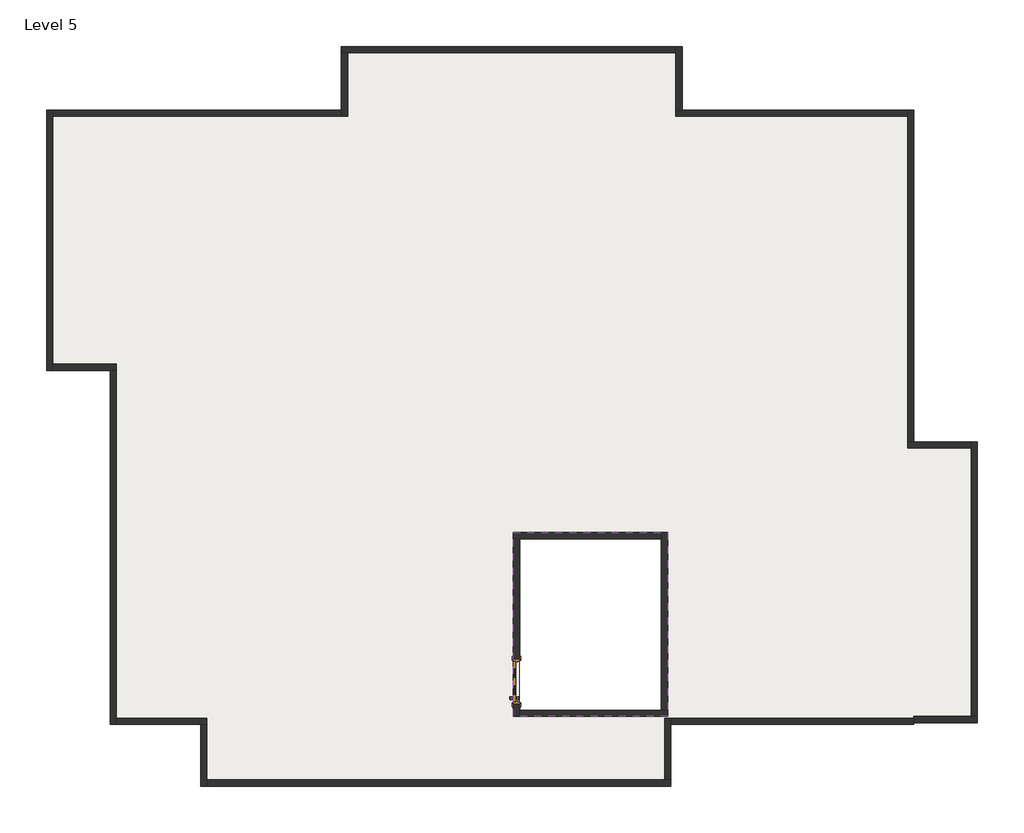
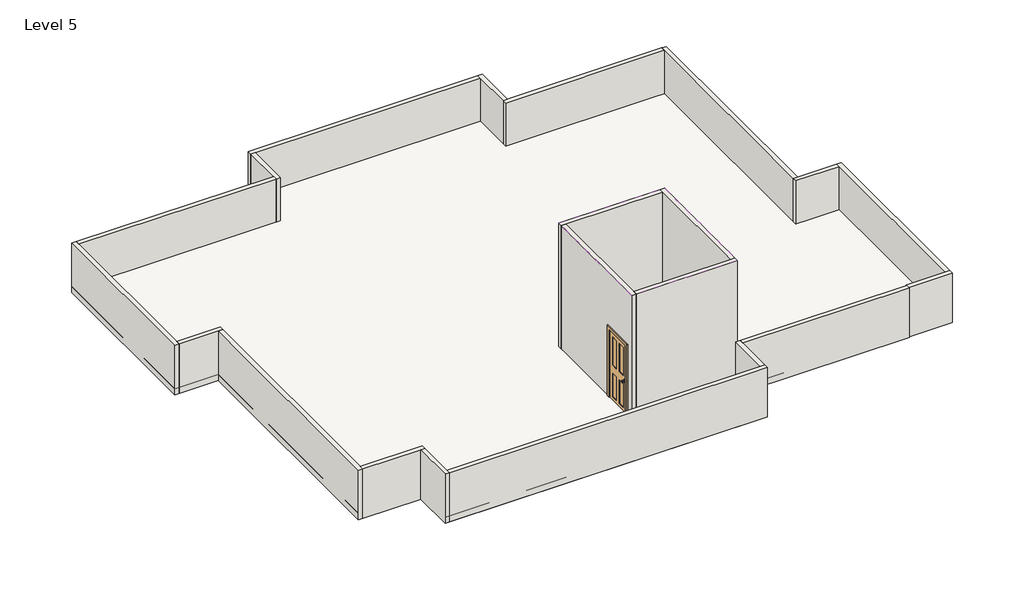
# One storey: 21 walls, 1 covering, 1 door, 1 slab.
"""IFC4 building model written with IfcOpenShell, lengths in millimetres."""

from ifc_helpers import new_model, si_unit, frame, origin, place, context, project, spatial, polyline, outline, extrude, faceted_brep, transform, mapped, element, save
from components import door_7e1124f1

model = new_model("IFC4")

# Units and contexts
model_context = context("Model", 3, world=origin())
ifc_project = project(units=[si_unit("LENGTHUNIT", "METRE", prefix="MILLI")], contexts=[model_context])

# Site, building, storey
site = spatial("IfcSite", under=ifc_project)
building = spatial("IfcBuilding", under=site)
storey = spatial("IfcBuildingStorey", under=building, Name="Level 5", Elevation=12801.6)

# Covering
placement = place(None, origin())
element("IfcCovering", 1, ObjectType="Plain", at=placement, inside=storey, context=model_context, shape_type="SweptSolid", body=[
    extrude(outline(polyline([(-9375.9794909, -1406.3618509), (-9375.9794909, -4352.7618509), (-11843.7794909, -4352.7618509), (-11843.7794909, -1406.3618509), (-9375.9794909, -1406.3618509)])), frame((0.0, 0.0, 16002.0), z_axis=(0.0, 0.0, 1.0), x_axis=(1.0, 0.0, 0.0)), (0.0, 0.0, 1.0), 57.0),
])

# Door
door_shape = door_7e1124f1(model_context)
element("IfcDoor", 2, ObjectType="M_Door-Interior-Single-4_Panel-Wood : 2'2\"", at=placement, inside=storey, context=model_context, shape_type="MappedRepresentation", body=[
    mapped(door_shape, transform((-11796.1544909, -3794.3618509, 12801.6), x_axis=(0.0, 1.0, 0.0), y_axis=(-1.0, 0.0, 0.0), z_axis=(0.0, 0.0, 1.0))),
])

# Slab
element("IfcSlab", 3, ObjectType="Generic 150mm", at=placement, inside=storey, context=model_context, shape_type="SweptSolid", body=[
    extrude(outline(polyline([(-18291.3794909, 1184.4381491), (-19307.3794909, 1184.4381491), (-19307.3794909, 5350.0381491), (-14596.2721539, 5350.0381491), (-14596.2721539, 6366.0381491), (-9142.3367869, 6366.0381491), (-9142.3367869, 5350.0381491), (-5438.9794909, 5350.0381491), (-5438.9794909, 41.4381491), (-4422.9794909, 41.4381491), (-4422.9794909, -4454.3618509), (-5438.9794909, -4454.3618509), (-5438.9794909, -4479.7618509), (-9325.1794909, -4479.7618509), (-9325.1794909, -5470.3618509), (-16843.5794909, -5470.3618509), (-16843.5794909, -4479.7618509), (-18291.3794909, -4479.7618509), (-18291.3794909, 1184.4381491)]), holes=[polyline([(-11738.1794909, -1507.9618509), (-11738.1794909, -4251.1618509), (-9477.5794909, -4251.1618509), (-9477.5794909, -1507.9618509), (-11738.1794909, -1507.9618509)])]), frame((0.0, 0.0, 12804.0), z_axis=(0.0, 0.0, 1.0), x_axis=(1.0, 0.0, 0.0)), (0.0, 0.0, 1.0), 150.0),
])

# Walls
element("IfcWall", 4, ObjectType="Generic - 4\"", at=placement, inside=storey, context=model_context, shape_type="Brep", body=[
    faceted_brep([(-19307.3794909, 5350.0381491, 12801.6), (-19307.3794909, 1184.4381491, 12801.6), (-19307.3794909, 1184.4381491, 14020.8), (-19307.3794909, 5350.0381491, 14020.8), (-19205.7794909, 5350.0381491, 12801.6), (-19205.7794909, 5350.0381491, 14020.8), (-19205.7794909, 5248.4381491, 14020.8), (-19205.7794909, 1286.0381491, 14020.8), (-19205.7794909, 1184.4381491, 14020.8), (-19205.7794909, 1184.4381491, 12801.6), (-19205.7794909, 1286.0381491, 12801.6), (-19205.7794909, 5248.4381491, 12801.6)], [[[0, 1, 2, 3]], [[4, 5, 6, 7, 8, 9, 10, 11]], [[1, 0, 4, 11, 10, 9]], [[3, 2, 8, 7, 6, 5]], [[2, 1, 9, 8]], [[0, 3, 5, 4]]]),
])
element("IfcWall", 5, ObjectType="Generic - 4\"", at=placement, inside=storey, context=model_context, shape_type="Brep", body=[
    faceted_brep([(-19205.7794909, 1184.4381491, 12801.6), (-18291.3794909, 1184.4381491, 12801.6), (-18189.7794909, 1184.4381491, 12801.6), (-18189.7794909, 1184.4381491, 14020.8), (-18291.3794909, 1184.4381491, 14020.8), (-19205.7794909, 1184.4381491, 14020.8), (-19205.7794909, 1286.0381491, 12801.6), (-19205.7794909, 1286.0381491, 14020.8), (-18189.7794909, 1286.0381491, 14020.8), (-18189.7794909, 1286.0381491, 12801.6)], [[[0, 1, 2, 3, 4, 5]], [[6, 7, 8, 9]], [[2, 1, 0, 6, 9]], [[5, 4, 3, 8, 7]], [[0, 5, 7, 6]], [[3, 2, 9, 8]]]),
])
element("IfcWall", 6, ObjectType="Generic - 4\"", at=placement, inside=storey, context=model_context, shape_type="Brep", body=[
    faceted_brep([(-18291.3794909, 1184.4381491, 12801.6), (-18291.3794909, -4479.7618509, 12801.6), (-18291.3794909, -4479.7618509, 14020.8), (-18291.3794909, 1184.4381491, 14020.8), (-18189.7794909, 1184.4381491, 12801.6), (-18189.7794909, 1184.4381491, 14020.8), (-18189.7794909, -4378.1618509, 14020.8), (-18189.7794909, -4479.7618509, 14020.8), (-18189.7794909, -4479.7618509, 12801.6), (-18189.7794909, -4378.1618509, 12801.6)], [[[0, 1, 2, 3]], [[4, 5, 6, 7, 8, 9]], [[1, 0, 4, 9, 8]], [[3, 2, 7, 6, 5]], [[0, 3, 5, 4]], [[2, 1, 8, 7]]]),
])
element("IfcWall", 7, ObjectType="Generic - 4\"", at=placement, inside=storey, context=model_context, shape_type="Brep", body=[
    faceted_brep([(-18189.7794909, -4479.7618509, 12801.6), (-16843.5794909, -4479.7618509, 12801.6), (-16741.9794909, -4479.7618509, 12801.6), (-16741.9794909, -4479.7618509, 14020.8), (-16843.5794909, -4479.7618509, 14020.8), (-18189.7794909, -4479.7618509, 14020.8), (-18189.7794909, -4378.1618509, 12801.6), (-18189.7794909, -4378.1618509, 14020.8), (-16741.9794909, -4378.1618509, 14020.8), (-16741.9794909, -4378.1618509, 12801.6)], [[[0, 1, 2, 3, 4, 5]], [[6, 7, 8, 9]], [[2, 1, 0, 6, 9]], [[5, 4, 3, 8, 7]], [[0, 5, 7, 6]], [[3, 2, 9, 8]]]),
])
element("IfcWall", 8, ObjectType="Generic - 4\"", at=placement, inside=storey, context=model_context, shape_type="Brep", body=[
    faceted_brep([(-16843.5794909, -4479.7618509, 12801.6), (-16843.5794909, -5470.3618509, 12801.6), (-16843.5794909, -5470.3618509, 14020.8), (-16843.5794909, -4479.7618509, 14020.8), (-16741.9794909, -4479.7618509, 12801.6), (-16741.9794909, -4479.7618509, 14020.8), (-16741.9794909, -5368.7618509, 14020.8), (-16741.9794909, -5470.3618509, 14020.8), (-16741.9794909, -5470.3618509, 12801.6), (-16741.9794909, -5368.7618509, 12801.6)], [[[0, 1, 2, 3]], [[4, 5, 6, 7, 8, 9]], [[1, 0, 4, 9, 8]], [[3, 2, 7, 6, 5]], [[0, 3, 5, 4]], [[2, 1, 8, 7]]]),
])
element("IfcWall", 9, ObjectType="Generic - 4\"", at=placement, inside=storey, context=model_context, shape_type="Brep", body=[
    faceted_brep([(-16741.9794909, -5470.3618509, 12801.6), (-9325.1794909, -5470.3618509, 12801.6), (-9325.1794909, -5470.3618509, 14020.8), (-16741.9794909, -5470.3618509, 14020.8), (-16741.9794909, -5368.7618509, 12801.6), (-16741.9794909, -5368.7618509, 14020.8), (-9426.7794909, -5368.7618509, 14020.8), (-9325.1794909, -5368.7618509, 14020.8), (-9325.1794909, -5368.7618509, 12801.6), (-9426.7794909, -5368.7618509, 12801.6)], [[[0, 1, 2, 3]], [[4, 5, 6, 7, 8, 9]], [[1, 0, 4, 9, 8]], [[3, 2, 7, 6, 5]], [[0, 3, 5, 4]], [[2, 1, 8, 7]]]),
])
element("IfcWall", 10, ObjectType="Generic - 4\"", at=placement, inside=storey, context=model_context, shape_type="Brep", body=[
    faceted_brep([(-9325.1794909, -5368.7618509, 12801.6), (-9325.1794909, -4479.7618509, 12801.6), (-9325.1794909, -4378.1618509, 12801.6), (-9325.1794909, -4378.1618509, 14020.8), (-9325.1794909, -4479.7618509, 14020.8), (-9325.1794909, -5368.7618509, 14020.8), (-9426.7794909, -5368.7618509, 12801.6), (-9426.7794909, -5368.7618509, 14020.8), (-9426.7794909, -4378.1618509, 14020.8), (-9426.7794909, -4378.1618509, 12801.6)], [[[0, 1, 2, 3, 4, 5]], [[6, 7, 8, 9]], [[2, 1, 0, 6, 9]], [[5, 4, 3, 8, 7]], [[0, 5, 7, 6]], [[3, 2, 9, 8]]]),
])
element("IfcWall", 11, ObjectType="Generic - 4\"", at=placement, inside=storey, context=model_context, shape_type="Brep", body=[
    faceted_brep([(-9325.1794909, -4479.7618509, 12801.6), (-5438.9794909, -4479.7618509, 12801.6), (-5438.9794909, -4479.7618509, 14020.8), (-9325.1794909, -4479.7618509, 14020.8), (-9325.1794909, -4378.1618509, 12801.6), (-9325.1794909, -4378.1618509, 14020.8), (-5438.9794909, -4378.1618509, 14020.8), (-5438.9794909, -4378.1618509, 12801.6), (-5438.9794909, -4454.3618509, 12801.6), (-5438.9794909, -4454.3618509, 14020.8)], [[[0, 1, 2, 3]], [[4, 5, 6, 7]], [[1, 0, 4, 7, 8]], [[2, 1, 8, 7, 6, 9]], [[3, 2, 9, 6, 5]], [[0, 3, 5, 4]]]),
])
element("IfcWall", 12, ObjectType="Generic - 4\"", at=placement, inside=storey, context=model_context, shape_type="Brep", body=[
    faceted_brep([(-5438.9794909, -4454.3618509, 12801.6), (-4422.9794909, -4454.3618509, 12801.6), (-4422.9794909, -4454.3618509, 14020.8), (-5438.9794909, -4454.3618509, 14020.8), (-5438.9794909, -4352.7618509, 12801.6), (-5438.9794909, -4352.7618509, 14020.8), (-4524.5794909, -4352.7618509, 14020.8), (-4422.9794909, -4352.7618509, 14020.8), (-4422.9794909, -4352.7618509, 12801.6), (-4524.5794909, -4352.7618509, 12801.6), (-5438.9794909, -4378.1618509, 12801.6), (-5438.9794909, -4378.1618509, 14020.8)], [[[0, 1, 2, 3]], [[4, 5, 6, 7, 8, 9]], [[1, 0, 10, 4, 9, 8]], [[3, 2, 7, 6, 5, 11]], [[0, 3, 11, 5, 4, 10]], [[2, 1, 8, 7]]]),
])
element("IfcWall", 13, ObjectType="Generic - 4\"", at=placement, inside=storey, context=model_context, shape_type="Brep", body=[
    faceted_brep([(-4422.9794909, -4352.7618509, 12801.6), (-4422.9794909, 41.4381491, 12801.6), (-4422.9794909, 41.4381491, 14020.8), (-4422.9794909, -4352.7618509, 14020.8), (-4524.5794909, -4352.7618509, 12801.6), (-4524.5794909, -4352.7618509, 14020.8), (-4524.5794909, -60.1618509, 14020.8), (-4524.5794909, 41.4381491, 14020.8), (-4524.5794909, 41.4381491, 12801.6), (-4524.5794909, -60.1618509, 12801.6)], [[[0, 1, 2, 3]], [[4, 5, 6, 7, 8, 9]], [[1, 0, 4, 9, 8]], [[3, 2, 7, 6, 5]], [[0, 3, 5, 4]], [[2, 1, 8, 7]]]),
])
element("IfcWall", 14, ObjectType="Generic - 4\"", at=placement, inside=storey, context=model_context, shape_type="Brep", body=[
    faceted_brep([(-4524.5794909, 41.4381491, 12801.6), (-5438.9794909, 41.4381491, 12801.6), (-5540.5794909, 41.4381491, 12801.6), (-5540.5794909, 41.4381491, 14020.8), (-5438.9794909, 41.4381491, 14020.8), (-4524.5794909, 41.4381491, 14020.8), (-4524.5794909, -60.1618509, 12801.6), (-4524.5794909, -60.1618509, 14020.8), (-5540.5794909, -60.1618509, 14020.8), (-5540.5794909, -60.1618509, 12801.6)], [[[0, 1, 2, 3, 4, 5]], [[6, 7, 8, 9]], [[2, 1, 0, 6, 9]], [[5, 4, 3, 8, 7]], [[0, 5, 7, 6]], [[3, 2, 9, 8]]]),
])
element("IfcWall", 15, ObjectType="Generic - 4\"", at=placement, inside=storey, context=model_context, shape_type="Brep", body=[
    faceted_brep([(-5438.9794909, 41.4381491, 12801.6), (-5438.9794909, 5350.0381491, 12801.6), (-5438.9794909, 5350.0381491, 14020.8), (-5438.9794909, 41.4381491, 14020.8), (-5540.5794909, 41.4381491, 12801.6), (-5540.5794909, 41.4381491, 14020.8), (-5540.5794909, 5248.4381491, 14020.8), (-5540.5794909, 5350.0381491, 14020.8), (-5540.5794909, 5350.0381491, 12801.6), (-5540.5794909, 5248.4381491, 12801.6)], [[[0, 1, 2, 3]], [[4, 5, 6, 7, 8, 9]], [[1, 0, 4, 9, 8]], [[3, 2, 7, 6, 5]], [[0, 3, 5, 4]], [[2, 1, 8, 7]]]),
])
element("IfcWall", 16, ObjectType="Generic - 4\"", at=placement, inside=storey, context=model_context, shape_type="Brep", body=[
    faceted_brep([(-5540.5794909, 5350.0381491, 12801.6), (-9142.3367869, 5350.0381491, 12801.6), (-9243.9367869, 5350.0381491, 12801.6), (-9243.9367869, 5350.0381491, 14020.8), (-9142.3367869, 5350.0381491, 14020.8), (-5540.5794909, 5350.0381491, 14020.8), (-5540.5794909, 5248.4381491, 12801.6), (-5540.5794909, 5248.4381491, 14020.8), (-9243.9367869, 5248.4381491, 14020.8), (-9243.9367869, 5248.4381491, 12801.6)], [[[0, 1, 2, 3, 4, 5]], [[6, 7, 8, 9]], [[2, 1, 0, 6, 9]], [[5, 4, 3, 8, 7]], [[0, 5, 7, 6]], [[3, 2, 9, 8]]]),
])
element("IfcWall", 17, ObjectType="Generic - 4\"", at=placement, inside=storey, context=model_context, shape_type="Brep", body=[
    faceted_brep([(-9142.3367869, 5350.0381491, 12801.6), (-9142.3367869, 6366.0381491, 12801.6), (-9142.3367869, 6366.0381491, 14020.8), (-9142.3367869, 5350.0381491, 14020.8), (-9243.9367869, 5350.0381491, 12801.6), (-9243.9367869, 5350.0381491, 14020.8), (-9243.9367869, 6264.4381491, 14020.8), (-9243.9367869, 6366.0381491, 14020.8), (-9243.9367869, 6366.0381491, 12801.6), (-9243.9367869, 6264.4381491, 12801.6)], [[[0, 1, 2, 3]], [[4, 5, 6, 7, 8, 9]], [[1, 0, 4, 9, 8]], [[3, 2, 7, 6, 5]], [[0, 3, 5, 4]], [[2, 1, 8, 7]]]),
])
element("IfcWall", 18, ObjectType="Generic - 4\"", at=placement, inside=storey, context=model_context, shape_type="Brep", body=[
    faceted_brep([(-9243.9367869, 6366.0381491, 12801.6), (-14596.2721539, 6366.0381491, 12801.6), (-14596.2721539, 6366.0381491, 14020.8), (-9243.9367869, 6366.0381491, 14020.8), (-9243.9367869, 6264.4381491, 12801.6), (-9243.9367869, 6264.4381491, 14020.8), (-14494.6721539, 6264.4381491, 14020.8), (-14596.2721539, 6264.4381491, 14020.8), (-14596.2721539, 6264.4381491, 12801.6), (-14494.6721539, 6264.4381491, 12801.6)], [[[0, 1, 2, 3]], [[4, 5, 6, 7, 8, 9]], [[1, 0, 4, 9, 8]], [[3, 2, 7, 6, 5]], [[0, 3, 5, 4]], [[2, 1, 8, 7]]]),
])
element("IfcWall", 19, ObjectType="Generic - 4\"", at=placement, inside=storey, context=model_context, shape_type="Brep", body=[
    faceted_brep([(-14596.2721539, 6264.4381491, 12801.6), (-14596.2721539, 5350.0381491, 12801.6), (-14596.2721539, 5248.4381491, 12801.6), (-14596.2721539, 5248.4381491, 14020.8), (-14596.2721539, 5350.0381491, 14020.8), (-14596.2721539, 6264.4381491, 14020.8), (-14494.6721539, 6264.4381491, 12801.6), (-14494.6721539, 6264.4381491, 14020.8), (-14494.6721539, 5248.4381491, 14020.8), (-14494.6721539, 5248.4381491, 12801.6)], [[[0, 1, 2, 3, 4, 5]], [[6, 7, 8, 9]], [[2, 1, 0, 6, 9]], [[5, 4, 3, 8, 7]], [[0, 5, 7, 6]], [[3, 2, 9, 8]]]),
])
element("IfcWall", 20, ObjectType="Generic - 4\"", at=placement, inside=storey, context=model_context, shape_type="SweptSolid", body=[
    extrude(outline(polyline([(-19205.7794909, 5350.0381491), (-14596.2721539, 5350.0381491), (-14596.2721539, 5248.4381491), (-19205.7794909, 5248.4381491), (-19205.7794909, 5350.0381491)])), frame((0.0, 0.0, 12801.6), z_axis=(0.0, 0.0, 1.0), x_axis=(1.0, 0.0, 0.0)), (0.0, 0.0, 1.0), 1219.2),
])
element("IfcWall", 21, ObjectType="Generic - 4\"", at=placement, inside=storey, context=model_context, shape_type="Brep", body=[
    faceted_brep([(-9375.9794909, -4251.1618509, 12801.6), (-9477.5794909, -4251.1618509, 12801.6), (-11742.1794909, -4251.1618509, 12801.6), (-11742.1794909, -4251.1618509, 16002.0), (-9477.5794909, -4251.1618509, 16002.0), (-9375.9794909, -4251.1618509, 16002.0), (-9375.9794909, -4352.7618509, 12801.6), (-9375.9794909, -4352.7618509, 16002.0), (-11742.1794909, -4352.7618509, 16002.0), (-11742.1794909, -4352.7618509, 12801.6)], [[[0, 1, 2, 3, 4, 5]], [[6, 7, 8, 9]], [[2, 1, 0, 6, 9]], [[5, 4, 3, 8, 7]], [[0, 5, 7, 6]], [[3, 2, 9, 8]]]),
])
element("IfcWall", 22, ObjectType="Generic - 4\"", at=placement, inside=storey, context=model_context, shape_type="Brep", body=[
    faceted_brep([(-9477.5794909, -1406.3618509, 12801.6), (-9477.5794909, -1507.9618509, 12801.6), (-9477.5794909, -4251.1618509, 12801.6), (-9477.5794909, -4251.1618509, 16002.0), (-9477.5794909, -1507.9618509, 16002.0), (-9477.5794909, -1406.3618509, 16002.0), (-9375.9794909, -1406.3618509, 12801.6), (-9375.9794909, -1406.3618509, 16002.0), (-9375.9794909, -4251.1618509, 16002.0), (-9375.9794909, -4251.1618509, 12801.6)], [[[0, 1, 2, 3, 4, 5]], [[6, 7, 8, 9]], [[2, 1, 0, 6, 9]], [[5, 4, 3, 8, 7]], [[0, 5, 7, 6]], [[3, 2, 9, 8]]]),
])
element("IfcWall", 23, ObjectType="Generic - 4\"", at=placement, inside=storey, context=model_context, shape_type="Brep", body=[
    faceted_brep([(-11843.7794909, -1507.9618509, 12801.6), (-11742.1794909, -1507.9618509, 12801.6), (-9477.5794909, -1507.9618509, 12801.6), (-9477.5794909, -1507.9618509, 16002.0), (-11742.1794909, -1507.9618509, 16002.0), (-11843.7794909, -1507.9618509, 16002.0), (-11843.7794909, -1406.3618509, 12801.6), (-11843.7794909, -1406.3618509, 16002.0), (-9477.5794909, -1406.3618509, 16002.0), (-9477.5794909, -1406.3618509, 12801.6)], [[[0, 1, 2, 3, 4, 5]], [[6, 7, 8, 9]], [[2, 1, 0, 6, 9]], [[5, 4, 3, 8, 7]], [[0, 5, 7, 6]], [[3, 2, 9, 8]]]),
])
element("IfcWall", 24, ObjectType="Generic - 4\"", at=placement, inside=storey, context=model_context, shape_type="Brep", body=[
    faceted_brep([(-11742.1794909, -1507.9618509, 16002.0), (-11742.1794909, -4251.1618509, 16002.0), (-11742.1794909, -4352.7618509, 16002.0), (-11742.1794909, -4352.7618509, 12801.6), (-11742.1794909, -4251.1618509, 12801.6), (-11742.1794909, -4149.5618509, 12801.6), (-11742.1794909, -4149.5618509, 14655.4), (-11742.1794909, -3439.1618509, 14655.4), (-11742.1794909, -3439.1618509, 12801.6), (-11742.1794909, -1507.9618509, 12801.6), (-11843.7794909, -4352.7618509, 16002.0), (-11843.7794909, -1507.9618509, 16002.0), (-11843.7794909, -1507.9618509, 12801.6), (-11843.7794909, -3439.1618509, 12801.6), (-11843.7794909, -3439.1618509, 14655.4), (-11843.7794909, -4149.5618509, 14655.4), (-11843.7794909, -4149.5618509, 12801.6), (-11843.7794909, -4352.7618509, 12801.6)], [[[0, 1, 2, 3, 4, 5, 6, 7, 8, 9]], [[10, 11, 12, 13, 14, 15, 16, 17]], [[3, 17, 16, 5, 4]], [[12, 9, 8, 13]], [[2, 1, 0, 11, 10]], [[3, 2, 10, 17]], [[0, 9, 12, 11]], [[7, 14, 13, 8]], [[15, 6, 5, 16]], [[6, 15, 14, 7]]]),
])

save(model, "model.ifc")

# Revit data of these elements
# Type "Plain"
#   built-in parameter 1002203 = 1 (stored number, unit not read)
#   built-in parameter 1002202 = 1 (stored number, unit not read)
#   Layers, outside or top first: 0' - 1.77165" "Metal Stud Layer" (function 1); 0' - 0.47244" "Gypsum Wall Board" (function 1)
# Type "M_Door-Interior-Single-4_Panel-Wood : 2'2\""
#   Type Mark = "43"
#   Assembly Code = "C1020300"
#   Analytic Construction = "Wooden"
#   Top Rail = 0' - 4.72441"
#   Thickness = 0' - 1.37795"
#   Thermal Resistance (R) = 0.455703 (m²·K)/W
#   Swing Angle [instance default] = 90.00°
#   Stiles = 0' - 4.72441"
#   Rough Width = 2' - 3.9685"
#   Rough Height = 6' - 0.98425"
#   Mullion = 0' - 4.52756"
#   Lock Rail = 0' - 7.87402"
#   Height = 6' - 0"
#   Width = 2' - 2"
#   Heat Transfer Coefficient (U) = 2.19465 W/(m²·K)
#   Bottom Rail = 0' - 9.05512"
#   Trim Material = Cherry
#   Panel Material = Cherry
#   Frame Material = Cherry
#   Door Handle Material = Aluminum
#   Visual Light Transmittance = 0
#   Solar Heat Gain Coefficient = 0
#   Wall Closure = (empty or 0)
#   Function = (empty or 0)
# Type "Generic 150mm"
#   Function = 0
#   Layers, outside or top first: 0' - 5.90551" no material (function 1)
# Type "Generic - 4\""
#   Layers, outside or top first: 0' - 4" no material (function 1)
# Element 1 (IfcCovering, "Plain")
#   Height Offset From Level = 10' - 6"
#   Phase Created = New Construction
#   Materials on its faces: "Gypsum Wall Board", "Metal Stud Layer"
# Element 2 (IfcDoor, "M_Door-Interior-Single-4_Panel-Wood : 2'2\"")
#   Swing Angle = 90.00°
#   Phase Created = New Construction
#   Materials on its faces: "Cherry", "Aluminum"
# Element 3 (IfcSlab, "Generic 150mm")
#   Height Offset From Level = 0' - 6"
#   Phase Created = New Construction
#   Materials on its faces: "Default Floor", "Concrete, Cast-in-Place, Gray"
# Elements 4, 5, 6, 7, 8, 9, 12, 13, 14, 15, 16, 17, 18, 19 (IfcWall, "Generic - 4\"")
#   Top Offset = 0' - 0"
#   Base Offset = 0' - 0"
#   Unconnected Height = 4' - 0"
#   wall height = 4' - 0"
#   Phase Created = New Construction
#   Base Constraint = Level 5
#   Materials on its faces: "WALL2", "Default Wall"
# Elements 10, 11, 20 (IfcWall, "Generic - 4\"")
#   Top Offset = 0' - 0"
#   Base Offset = 0' - 0"
#   Unconnected Height = 4' - 0"
#   wall height = 4' - 0"
#   Phase Created = New Construction
#   Base Constraint = Level 5
#   Materials on its faces: "Default Wall", "WALL2"
# Elements 21, 22, 23, 24 (IfcWall, "Generic - 4\"")
#   Top Offset = 0' - 0"
#   Base Offset = 0' - 0"
#   Unconnected Height = 10' - 6"
#   wall height = 10' - 6"
#   Phase Created = New Construction
#   Base Constraint = Level 5
#   Materials on its faces: "Default Wall", "WALL2"
# Materials
#   "Metal Stud Layer": class "Metal", colour RGB 127 127 127, transparency 0, Description = "Light gauge steel framing, thermal air layer", Cost = 0
#   "Gypsum Wall Board": class "Generic", colour RGB 249 249 249, transparency 0, Description = "Gypsum Wall Board", Cost = 0
#   "Cherry": class "Wood", colour RGB 226 177 128, transparency 0, Description = "Prunus Serotina", Cost = 0
#   "Aluminum": class "Metal", colour RGB 247 247 247, transparency 0, Description = "Aluminum 6061", Cost = 0
#   "Default Floor": colour RGB 127 127 127, transparency 0, Cost = 0
#   "Concrete, Cast-in-Place, Gray": class "Concrete", colour RGB 192 192 192, transparency 0, Description = "Cast-in-place concrete", Cost = 0
#   "WALL2": class "Generic", colour RGB 120 120 120, transparency 0, Cost = 0
#   "Default Wall": colour RGB 128 128 128, transparency 0, Cost = 0
